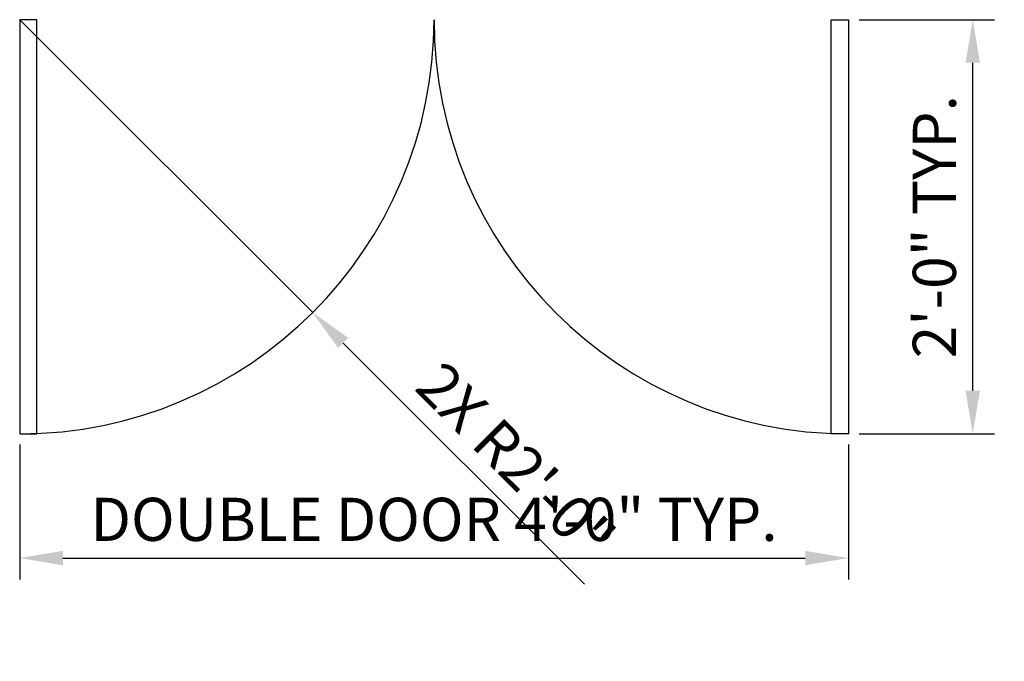
# Model space of a CAD drawing. Units: inches. Extents: x 877 to 2164, y 771 to 1603.
# Tile 5 of 6: x 1951 to 2008, y 1087 to 1124. Entities that reach past the tile are written whole.
import ezdxf

# ---------------------------------------------------------------- set-up
doc = ezdxf.new("R2010")
doc.units = ezdxf.units.IN
doc.layers.add('A-ANNO-DIMS', color=2, linetype='Continuous', lineweight=18)
doc.layers.add('A-DOOR', color=5, linetype='Continuous', lineweight=25)
doc.styles.get("Standard").update_dxf_attribs({"font": 'arial.ttf'})
doc.dimstyles.new('ISO-25', dxfattribs={"dimtxt": 2.5, "dimasz": 2.5, "dimexe": 1.25, "dimexo": 0.625, "dimtad": 1, "dimdec": 0, "dimlunit": 4, "dimtxsty": 'Standard', "dimcen": 2.5, "dimadec": 0, "dimazin": 0, "dimtfac": 1, "dimtdec": 0, "dimtmove": 0, "dimatfit": 3, "dimfxl": 1, "dimarcsym": 0})

# ---------------------------------------------------------------- blocks, each defined once
blk = doc.blocks.new('DOOR-DOUBLE-48IN')
for points in [[(0, 0), (1, 0), (1, 24), (0, 24)], [(48, 0), (47, 0), (47, 24), (48, 24)]]:
    blk.add_lwpolyline(points, close=True)
for centre, start, end in [((0, 24), 270, 0), ((48, 24), 180, 270)]:
    blk.add_arc(centre, 24, start, end)
blk = doc.blocks.new('*D8')
at = {"layer": 'A-ANNO-DIMS', "color": 0, "lineweight": -2, "transparency": 16777216}
for p, q in [((1950.564, 1099.867), (1950.564, 1092.042)), ((1998.564, 1099.867), (1998.564, 1092.042)), ((1953.064, 1093.292), (1996.064, 1093.292))]:
    blk.add_line(p, q, dxfattribs=at)
at = {"layer": 'A-ANNO-DIMS', "color": 0, "transparency": 16777216}
for points in [[(1953.064, 1093.708), (1953.064, 1092.875), (1950.564, 1093.292)], [(1996.064, 1093.708), (1996.064, 1092.875), (1998.564, 1093.292)]]:
    blk.add_solid(points, dxfattribs=at)
at = {"layer": 'Defpoints', "color": 0, "transparency": 16777216}
for p in [(1950.564, 1100.492), (1998.564, 1100.492), (1998.564, 1093.292)]:
    blk.add_point(p, dxfattribs=at)
at = {"layer": 'A-ANNO-DIMS', "color": 0, "transparency": 16777216, "insert": (1974.564, 1095.21), "char_height": 2.5, "attachment_point": 5}
blk.add_mtext('DOUBLE DOOR 4\'-0" TYP.', dxfattribs=at)
blk = doc.blocks.new('*D9')
at = {"layer": 'A-ANNO-DIMS', "color": 0, "lineweight": -2, "transparency": 16777216}
for p, q in [((1999.189, 1124.492), (2007.014, 1124.492)), ((2005.764, 1102.992), (2005.764, 1121.992)), ((1999.189, 1100.492), (2007.014, 1100.492))]:
    blk.add_line(p, q, dxfattribs=at)
at = {"layer": 'A-ANNO-DIMS', "color": 0, "transparency": 16777216}
for points in [[(2005.348, 1121.992), (2006.181, 1121.992), (2005.764, 1124.492)], [(2005.348, 1102.992), (2006.181, 1102.992), (2005.764, 1100.492)]]:
    blk.add_solid(points, dxfattribs=at)
at = {"layer": 'Defpoints', "color": 0, "transparency": 16777216}
for p in [(1998.564, 1124.492), (2005.764, 1124.492), (1998.564, 1100.492)]:
    blk.add_point(p, dxfattribs=at)
at = {"layer": 'A-ANNO-DIMS', "color": 0, "transparency": 16777216, "insert": (2003.863, 1112.492), "char_height": 2.5, "attachment_point": 5, "rotation": 90}
blk.add_mtext('2\'-0" TYP.', dxfattribs=at)
blk = doc.blocks.new('*D48')
at = {"layer": 'A-ANNO-DIMS', "color": 0, "lineweight": -2, "transparency": 16777216}
for p, q in [((1950.564, 1124.492), (1967.535, 1107.521)), ((1983.269, 1091.787), (1969.303, 1105.753))]:
    blk.add_line(p, q, dxfattribs=at)
at = {"layer": 'A-ANNO-DIMS', "color": 0, "transparency": 16777216}
blk.add_solid([(1969.597, 1106.048), (1969.008, 1105.459), (1967.535, 1107.521)], dxfattribs=at)
at = {"layer": 'Defpoints', "color": 0, "transparency": 16777216}
for p in [(1950.564, 1124.492), (1967.535, 1107.521)]:
    blk.add_point(p, dxfattribs=at)
at = {"layer": 'A-ANNO-DIMS', "color": 0, "transparency": 16777216, "insert": (1979.062, 1098.683), "char_height": 2.5, "attachment_point": 5, "rotation": 315.0003}
blk.add_mtext('2X R2\'-0"', dxfattribs=at)

msp = doc.modelspace()

# ---------------------------------------------------------------- block references
at = {"layer": 'A-DOOR'}
msp.add_blockref('DOOR-DOUBLE-48IN', (1950.564, 1100.492), dxfattribs=at)

# ---------------------------------------------------------------- dimensions: what is measured, and where the dimension line sits
at = {"layer": 'A-ANNO-DIMS'}
dim = msp.add_radius_dim(center=(1950.564, 1124.492), mpoint=(1967.535, 1107.521), text='2X <>', dimstyle='ISO-25', override={"dimdec": 1, "dimlfac": 1, "dimrnd": 0, "dimzin": 1, "dimdsep": 46, "dimlunit": 4, "dimfrac": 2}, dxfattribs=at)
dim.commit()
dim.dimension.update_dxf_attribs({"geometry": '*D48', "text_midpoint": (1977.717, 1097.339), "dimtype": 164})
dim = msp.add_linear_dim(base=(2005.764, 1124.492), p1=(1998.564, 1100.492), p2=(1998.564, 1124.492), angle=90, text='<> TYP.', dimstyle='ISO-25', override={"dimdec": 1, "dimlfac": 1, "dimrnd": 0, "dimzin": 1, "dimdsep": 46, "dimlunit": 4, "dimfrac": 2}, dxfattribs=at)
dim.commit()
dim.dimension.update_dxf_attribs({"geometry": '*D9', "text_midpoint": (2003.863, 1112.492)})
dim = msp.add_linear_dim(base=(1998.564, 1093.292), p1=(1950.564, 1100.492), p2=(1998.564, 1100.492), text='DOUBLE DOOR <> TYP.', dimstyle='ISO-25', override={"dimdec": 1, "dimlfac": 1, "dimrnd": 0, "dimzin": 1, "dimdsep": 46, "dimlunit": 4, "dimfrac": 2}, dxfattribs=at)
dim.commit()
dim.dimension.update_dxf_attribs({"geometry": '*D8', "text_midpoint": (1974.564, 1095.21)})

doc.saveas('drawing.dxf')
